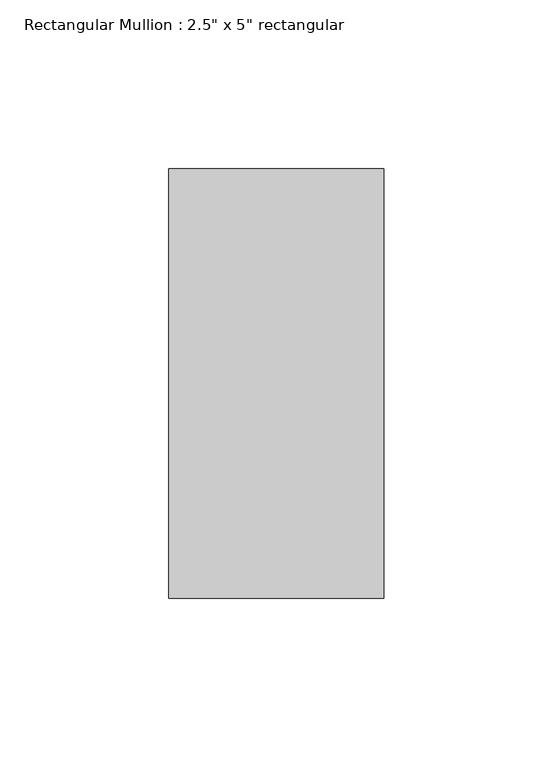
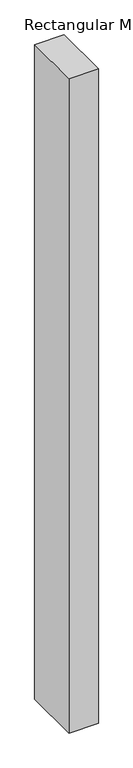
"""IFC4 building model written with IfcOpenShell, lengths in millimetres: member geometry."""

from ifc_helpers import new_model, si_unit, frame, origin, place, context, project, spatial, polyline, outline, extrude, source, transform, mapped, element, save


def member_c85333fa(model_context):
    return source(origin(), model_context, "Body", "SweptSolid", [
        extrude(outline(polyline([(0.0, 63.5), (0.0, -63.5), (-63.5, -63.5), (-63.5, 63.5), (0.0, 63.5)])), frame((0.0, 0.0, -1486.8504732), z_axis=(0.0, 0.0, 1.0), x_axis=(1.0, 0.0, 0.0)), (0.0, 0.0, 1.0), 1486.8504732),
    ])


if __name__ == "__main__":
    model = new_model("IFC4")
    model_context = context("Model", 3, world=origin())
    ifc_project = project(units=[si_unit("LENGTHUNIT", "METRE", prefix="MILLI")], contexts=[model_context])
    site = spatial("IfcSite", under=ifc_project)
    building = spatial("IfcBuilding", under=site)
    placement = place(None, origin())
    member_shape = member_c85333fa(model_context)
    element("IfcMember", 1, ObjectType="Rectangular Mullion : 2.5\" x 5\" rectangular", at=placement, inside=building, context=model_context, shape_type="MappedRepresentation", body=[
        mapped(member_shape, transform((0.0, 0.0, 0.0), x_axis=(1.0, 0.0, 0.0), y_axis=(0.0, 1.0, 0.0), z_axis=(0.0, 0.0, 1.0))),
    ])
    save(model, "model.ifc")

# Revit data of these elements
# Type "Rectangular Mullion : 2.5\" x 5\" rectangular"
#   built-in parameter 1007304 = 0.416667 (stored number, unit not read)
#   built-in parameter 1007301 = 0.104167 (stored number, unit not read)
#   built-in parameter 1007300 = 0.104167 (stored number, unit not read)
# Element 1 (IfcMember, "Rectangular Mullion : 2.5\" x 5\" rectangular")
#   Materials on its faces: "Aluminum"
# Materials
#   "Aluminum": class "Metal", colour RGB 247 247 247, transparency 0, Description = "Aluminum 6061", Cost = 0
